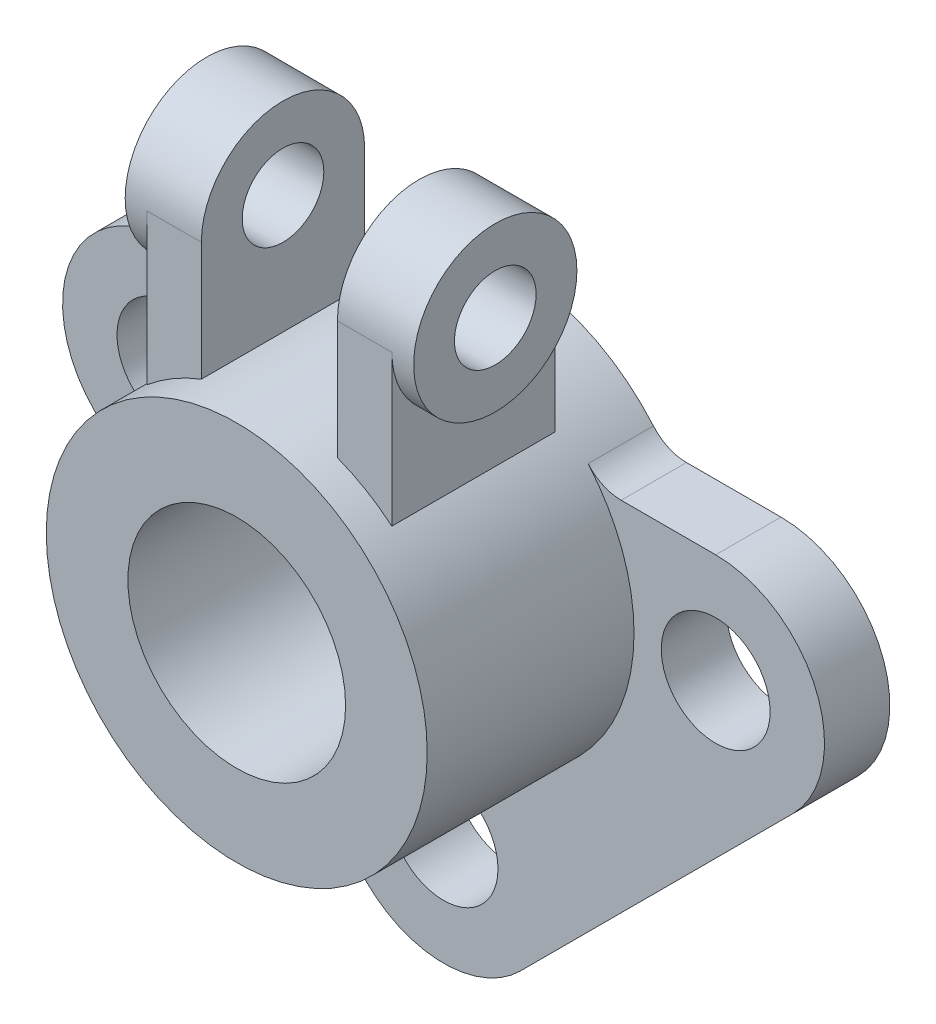
ISO-10303-21;
HEADER;
FILE_DESCRIPTION(('STEP AP214'),'2;1');
FILE_NAME('part.step','',(''),(''),'','','');
FILE_SCHEMA(('AUTOMOTIVE_DESIGN { 1 0 10303 214 1 1 1 1 }'));
ENDSEC;
DATA;
#1=APPLICATION_CONTEXT('core data for automotive mechanical design processes');
#2=APPLICATION_PROTOCOL_DEFINITION('international standard','automotive_design',2000,#1);
#3=PRODUCT_CONTEXT('',#1,'mechanical');
#4=PRODUCT('Part','Part','',(#3));
#5=PRODUCT_RELATED_PRODUCT_CATEGORY('part','',(#4));
#6=PRODUCT_DEFINITION_FORMATION('','',#4);
#7=PRODUCT_DEFINITION_CONTEXT('part definition',#1,'design');
#8=PRODUCT_DEFINITION('design','',#6,#7);
#9=PRODUCT_DEFINITION_SHAPE('','',#8);
#10=(LENGTH_UNIT() NAMED_UNIT(*) SI_UNIT(.MILLI.,.METRE.));
#11=(NAMED_UNIT(*) PLANE_ANGLE_UNIT() SI_UNIT($,.RADIAN.));
#12=(NAMED_UNIT(*) SI_UNIT($,.STERADIAN.) SOLID_ANGLE_UNIT());
#13=UNCERTAINTY_MEASURE_WITH_UNIT(LENGTH_MEASURE(1.E-05),#10,'distance_accuracy_value','');
#14=(GEOMETRIC_REPRESENTATION_CONTEXT(3) GLOBAL_UNCERTAINTY_ASSIGNED_CONTEXT((#13)) GLOBAL_UNIT_ASSIGNED_CONTEXT((#10,
#11,#12)) REPRESENTATION_CONTEXT('',''));
#15=CARTESIAN_POINT('',(0.,0.,0.));
#16=DIRECTION('',(0.,0.,1.));
#17=DIRECTION('',(1.,0.,0.));
#18=AXIS2_PLACEMENT_3D('',#15,#16,#17);
#19=CARTESIAN_POINT('',(-22.5,54.4714103742384,-21.));
#20=DIRECTION('',(1.,0.,0.));
#21=DIRECTION('',(0.,0.,-1.));
#22=AXIS2_PLACEMENT_3D('',#19,#20,#21);
#23=PLANE('',#22);
#24=CARTESIAN_POINT('',(-22.5,54.4714103742384,-21.));
#25=DIRECTION('',(1.,0.,0.));
#26=DIRECTION('',(0.,0.,-1.));
#27=AXIS2_PLACEMENT_3D('',#24,#25,#26);
#28=CIRCLE('',#27,15.);
#29=CARTESIAN_POINT('',(-22.5,54.4714103742384,-36.));
#30=VERTEX_POINT('',#29);
#31=CARTESIAN_POINT('',(-22.5,54.4714103742384,-6.00000000000001));
#32=VERTEX_POINT('',#31);
#33=EDGE_CURVE('E11',#30,#32,#28,.F.);
#34=ORIENTED_EDGE('',*,*,#33,.F.);
#35=DIRECTION('',(0.,1.,0.));
#36=VECTOR('',#35,1.);
#37=CARTESIAN_POINT('',(-22.5,54.4714103742384,-36.));
#38=LINE('',#37,#36);
#39=CARTESIAN_POINT('',(-22.5,26.809513236909,-36.));
#40=VERTEX_POINT('',#39);
#41=EDGE_CURVE('E168',#40,#30,#38,.T.);
#42=ORIENTED_EDGE('',*,*,#41,.F.);
#43=DIRECTION('',(0.,0.,1.));
#44=VECTOR('',#43,1.);
#45=CARTESIAN_POINT('',(-22.5,26.809513236909,-50.));
#46=LINE('',#45,#44);
#47=CARTESIAN_POINT('',(-22.5,26.809513236909,-6.00000000000001));
#48=VERTEX_POINT('',#47);
#49=EDGE_CURVE('E55',#48,#40,#46,.F.);
#50=ORIENTED_EDGE('',*,*,#49,.F.);
#51=DIRECTION('',(0.,-1.,0.));
#52=VECTOR('',#51,1.);
#53=CARTESIAN_POINT('',(-22.5,26.4714103742384,-6.00000000000001));
#54=LINE('',#53,#52);
#55=EDGE_CURVE('E166',#32,#48,#54,.T.);
#56=ORIENTED_EDGE('',*,*,#55,.F.);
#57=EDGE_LOOP('',(#34,#42,#50,#56));
#58=FACE_BOUND('',#57,.T.);
#59=ADVANCED_FACE('F43',(#58),#23,.F.);
#60=CARTESIAN_POINT('',(0.,0.,-50.));
#61=DIRECTION('',(0.,0.,1.));
#62=DIRECTION('',(1.,0.,0.));
#63=AXIS2_PLACEMENT_3D('',#60,#61,#62);
#64=CYLINDRICAL_SURFACE('',#63,35.);
#65=DIRECTION('',(0.,0.,1.));
#66=VECTOR('',#65,1.);
#67=CARTESIAN_POINT('',(22.5,26.809513236909,-50.));
#68=LINE('',#67,#66);
#69=CARTESIAN_POINT('',(22.5,26.809513236909,-6.));
#70=VERTEX_POINT('',#69);
#71=CARTESIAN_POINT('',(22.5,26.809513236909,-36.));
#72=VERTEX_POINT('',#71);
#73=EDGE_CURVE('E328',#70,#72,#68,.F.);
#74=ORIENTED_EDGE('',*,*,#73,.F.);
#75=CARTESIAN_POINT('',(0.,0.,-5.99999999999999));
#76=DIRECTION('',(0.,0.,-1.));
#77=DIRECTION('',(0.,1.,0.));
#78=AXIS2_PLACEMENT_3D('',#75,#76,#77);
#79=CIRCLE('',#78,35.);
#80=CARTESIAN_POINT('',(12.5,32.6917420765551,-6.));
#81=VERTEX_POINT('',#80);
#82=EDGE_CURVE('E324',#70,#81,#79,.F.);
#83=ORIENTED_EDGE('',*,*,#82,.T.);
#84=DIRECTION('',(0.,0.,1.));
#85=VECTOR('',#84,1.);
#86=CARTESIAN_POINT('',(12.5,32.6917420765551,-50.));
#87=LINE('',#86,#85);
#88=CARTESIAN_POINT('',(12.5,32.6917420765551,-36.));
#89=VERTEX_POINT('',#88);
#90=EDGE_CURVE('E320',#81,#89,#87,.F.);
#91=ORIENTED_EDGE('',*,*,#90,.T.);
#92=CARTESIAN_POINT('',(0.,0.,-36.));
#93=DIRECTION('',(0.,0.,1.));
#94=DIRECTION('',(0.,-1.,0.));
#95=AXIS2_PLACEMENT_3D('',#92,#93,#94);
#96=CIRCLE('',#95,35.);
#97=EDGE_CURVE('E318',#89,#72,#96,.F.);
#98=ORIENTED_EDGE('',*,*,#97,.T.);
#99=EDGE_LOOP('',(#74,#83,#91,#98));
#100=FACE_BOUND('',#99,.T.);
#101=CARTESIAN_POINT('',(0.,0.,-50.));
#102=DIRECTION('',(0.,0.,1.));
#103=DIRECTION('',(1.,0.,0.));
#104=AXIS2_PLACEMENT_3D('',#101,#102,#103);
#105=CIRCLE('',#104,35.);
#106=CARTESIAN_POINT('',(26.5628330475733,22.7906976744186,-50.));
#107=VERTEX_POINT('',#106);
#108=CARTESIAN_POINT('',(-26.5628330475733,22.7906976744186,-50.));
#109=VERTEX_POINT('',#108);
#110=EDGE_CURVE('E291',#107,#109,#105,.T.);
#111=ORIENTED_EDGE('',*,*,#110,.T.);
#112=DIRECTION('',(0.,0.,1.));
#113=VECTOR('',#112,1.);
#114=CARTESIAN_POINT('',(-26.5628330475733,22.7906976744186,-50.));
#115=LINE('',#114,#113);
#116=CARTESIAN_POINT('',(-26.5628330475733,22.7906976744186,-38.));
#117=VERTEX_POINT('',#116);
#118=EDGE_CURVE('E297',#109,#117,#115,.T.);
#119=ORIENTED_EDGE('',*,*,#118,.T.);
#120=CARTESIAN_POINT('',(0.,0.,-38.));
#121=DIRECTION('',(0.,0.,-1.));
#122=DIRECTION('',(1.,0.,0.));
#123=AXIS2_PLACEMENT_3D('',#120,#121,#122);
#124=CIRCLE('',#123,35.);
#125=CARTESIAN_POINT('',(26.5628330475733,22.7906976744186,-38.));
#126=VERTEX_POINT('',#125);
#127=EDGE_CURVE('E272',#126,#117,#124,.T.);
#128=ORIENTED_EDGE('',*,*,#127,.F.);
#129=DIRECTION('',(0.,0.,1.));
#130=VECTOR('',#129,1.);
#131=CARTESIAN_POINT('',(26.5628330475733,22.7906976744186,-50.));
#132=LINE('',#131,#130);
#133=EDGE_CURVE('E298',#126,#107,#132,.F.);
#134=ORIENTED_EDGE('',*,*,#133,.T.);
#135=EDGE_LOOP('',(#111,#119,#128,#134));
#136=FACE_BOUND('',#135,.T.);
#137=CARTESIAN_POINT('',(0.,0.,0.));
#138=DIRECTION('',(0.,0.,1.));
#139=DIRECTION('',(1.,0.,0.));
#140=AXIS2_PLACEMENT_3D('',#137,#138,#139);
#141=CIRCLE('',#140,35.);
#142=CARTESIAN_POINT('',(35.,0.,0.));
#143=VERTEX_POINT('',#142);
#144=EDGE_CURVE('E287',#143,#143,#141,.T.);
#145=ORIENTED_EDGE('',*,*,#144,.F.);
#146=EDGE_LOOP('',(#145));
#147=FACE_BOUND('',#146,.T.);
#148=CARTESIAN_POINT('',(0.,0.,-6.00000000000001));
#149=DIRECTION('',(0.,0.,1.));
#150=DIRECTION('',(0.,-1.,0.));
#151=AXIS2_PLACEMENT_3D('',#148,#149,#150);
#152=CIRCLE('',#151,35.);
#153=CARTESIAN_POINT('',(-12.5,32.6917420765551,-6.00000000000001));
#154=VERTEX_POINT('',#153);
#155=EDGE_CURVE('E64',#48,#154,#152,.F.);
#156=ORIENTED_EDGE('',*,*,#155,.F.);
#157=ORIENTED_EDGE('',*,*,#49,.T.);
#158=CARTESIAN_POINT('',(0.,0.,-36.));
#159=DIRECTION('',(0.,0.,-1.));
#160=DIRECTION('',(0.,1.,0.));
#161=AXIS2_PLACEMENT_3D('',#158,#159,#160);
#162=CIRCLE('',#161,35.);
#163=CARTESIAN_POINT('',(-12.5,32.6917420765551,-36.));
#164=VERTEX_POINT('',#163);
#165=EDGE_CURVE('E178',#164,#40,#162,.F.);
#166=ORIENTED_EDGE('',*,*,#165,.F.);
#167=DIRECTION('',(0.,0.,1.));
#168=VECTOR('',#167,1.);
#169=CARTESIAN_POINT('',(-12.5,32.6917420765551,-50.));
#170=LINE('',#169,#168);
#171=EDGE_CURVE('E333',#154,#164,#170,.F.);
#172=ORIENTED_EDGE('',*,*,#171,.F.);
#173=EDGE_LOOP('',(#156,#157,#166,#172));
#174=FACE_BOUND('',#173,.T.);
#175=ADVANCED_FACE('F385',(#100,#136,#147,#174),#64,.T.);
#176=CARTESIAN_POINT('',(22.5,54.4714103742384,-21.));
#177=DIRECTION('',(1.,0.,0.));
#178=DIRECTION('',(0.,0.,-1.));
#179=AXIS2_PLACEMENT_3D('',#176,#177,#178);
#180=PLANE('',#179);
#181=DIRECTION('',(0.,1.,0.));
#182=VECTOR('',#181,1.);
#183=CARTESIAN_POINT('',(22.5,26.4714103742384,-36.));
#184=LINE('',#183,#182);
#185=CARTESIAN_POINT('',(22.5,54.4714103742384,-36.));
#186=VERTEX_POINT('',#185);
#187=EDGE_CURVE('E197',#72,#186,#184,.T.);
#188=ORIENTED_EDGE('',*,*,#187,.T.);
#189=CARTESIAN_POINT('',(22.5,54.4714103742384,-21.));
#190=DIRECTION('',(1.,0.,0.));
#191=DIRECTION('',(0.,0.,-1.));
#192=AXIS2_PLACEMENT_3D('',#189,#190,#191);
#193=CIRCLE('',#192,15.);
#194=CARTESIAN_POINT('',(22.5,54.4714103742384,-6.00000000000001));
#195=VERTEX_POINT('',#194);
#196=EDGE_CURVE('E327',#186,#195,#193,.F.);
#197=ORIENTED_EDGE('',*,*,#196,.T.);
#198=DIRECTION('',(0.,-1.,0.));
#199=VECTOR('',#198,1.);
#200=CARTESIAN_POINT('',(22.5,54.4714103742384,-6.00000000000001));
#201=LINE('',#200,#199);
#202=EDGE_CURVE('E193',#195,#70,#201,.T.);
#203=ORIENTED_EDGE('',*,*,#202,.T.);
#204=ORIENTED_EDGE('',*,*,#73,.T.);
#205=EDGE_LOOP('',(#188,#197,#203,#204));
#206=FACE_BOUND('',#205,.T.);
#207=ADVANCED_FACE('F390',(#206),#180,.T.);
#208=CARTESIAN_POINT('',(0.,0.,-50.));
#209=DIRECTION('',(0.,0.,1.));
#210=DIRECTION('',(1.,0.,0.));
#211=AXIS2_PLACEMENT_3D('',#208,#209,#210);
#212=PLANE('',#211);
#213=CARTESIAN_POINT('',(50.,0.,-50.));
#214=DIRECTION('',(0.,0.,1.));
#215=DIRECTION('',(1.,0.,0.));
#216=AXIS2_PLACEMENT_3D('',#213,#214,#215);
#217=CIRCLE('',#216,10.);
#218=CARTESIAN_POINT('',(60.,0.,-50.));
#219=VERTEX_POINT('',#218);
#220=EDGE_CURVE('E211',#219,#219,#217,.T.);
#221=ORIENTED_EDGE('',*,*,#220,.T.);
#222=EDGE_LOOP('',(#221));
#223=FACE_BOUND('',#222,.T.);
#224=CARTESIAN_POINT('',(0.,-50.,-50.));
#225=DIRECTION('',(0.,0.,1.));
#226=DIRECTION('',(1.,0.,0.));
#227=AXIS2_PLACEMENT_3D('',#224,#225,#226);
#228=CIRCLE('',#227,10.);
#229=CARTESIAN_POINT('',(10.,-50.,-50.));
#230=VERTEX_POINT('',#229);
#231=EDGE_CURVE('E223',#230,#230,#228,.T.);
#232=ORIENTED_EDGE('',*,*,#231,.T.);
#233=EDGE_LOOP('',(#232));
#234=FACE_BOUND('',#233,.T.);
#235=CARTESIAN_POINT('',(-50.,0.,-50.));
#236=DIRECTION('',(0.,0.,1.));
#237=DIRECTION('',(1.,0.,0.));
#238=AXIS2_PLACEMENT_3D('',#235,#236,#237);
#239=CIRCLE('',#238,10.);
#240=CARTESIAN_POINT('',(-40.,0.,-50.));
#241=VERTEX_POINT('',#240);
#242=EDGE_CURVE('E227',#241,#241,#239,.T.);
#243=ORIENTED_EDGE('',*,*,#242,.T.);
#244=EDGE_LOOP('',(#243));
#245=FACE_BOUND('',#244,.T.);
#246=CARTESIAN_POINT('',(0.,0.,-50.));
#247=DIRECTION('',(0.,0.,1.));
#248=DIRECTION('',(1.,0.,0.));
#249=AXIS2_PLACEMENT_3D('',#246,#247,#248);
#250=CIRCLE('',#249,20.);
#251=CARTESIAN_POINT('',(20.,0.,-50.));
#252=VERTEX_POINT('',#251);
#253=EDGE_CURVE('E290',#252,#252,#250,.T.);
#254=ORIENTED_EDGE('',*,*,#253,.T.);
#255=EDGE_LOOP('',(#254));
#256=FACE_BOUND('',#255,.T.);
#257=ORIENTED_EDGE('',*,*,#110,.F.);
#258=CARTESIAN_POINT('',(32.6343377441614,28.,-50.));
#259=DIRECTION('',(0.,0.,1.));
#260=DIRECTION('',(1.,0.,0.));
#261=AXIS2_PLACEMENT_3D('',#258,#259,#260);
#262=CIRCLE('',#261,8.);
#263=CARTESIAN_POINT('',(32.6343377441614,20.,-50.));
#264=VERTEX_POINT('',#263);
#265=EDGE_CURVE('E314',#107,#264,#262,.T.);
#266=ORIENTED_EDGE('',*,*,#265,.T.);
#267=DIRECTION('',(-1.,0.,0.));
#268=VECTOR('',#267,1.);
#269=CARTESIAN_POINT('',(50.,20.,-50.));
#270=LINE('',#269,#268);
#271=CARTESIAN_POINT('',(50.,20.,-50.));
#272=VERTEX_POINT('',#271);
#273=EDGE_CURVE('E247',#272,#264,#270,.T.);
#274=ORIENTED_EDGE('',*,*,#273,.F.);
#275=CARTESIAN_POINT('',(50.,0.,-50.));
#276=DIRECTION('',(0.,0.,1.));
#277=DIRECTION('',(1.,0.,0.));
#278=AXIS2_PLACEMENT_3D('',#275,#276,#277);
#279=CIRCLE('',#278,20.);
#280=CARTESIAN_POINT('',(64.1421356237309,-14.142135623731,-50.));
#281=VERTEX_POINT('',#280);
#282=EDGE_CURVE('E244',#281,#272,#279,.T.);
#283=ORIENTED_EDGE('',*,*,#282,.F.);
#284=DIRECTION('',(0.707106781186547,0.707106781186548,0.));
#285=VECTOR('',#284,1.);
#286=CARTESIAN_POINT('',(64.142135623731,-14.1421356237309,-50.));
#287=LINE('',#286,#285);
#288=CARTESIAN_POINT('',(14.142135623731,-64.142135623731,-50.));
#289=VERTEX_POINT('',#288);
#290=EDGE_CURVE('E245',#289,#281,#287,.T.);
#291=ORIENTED_EDGE('',*,*,#290,.F.);
#292=CARTESIAN_POINT('',(0.,-50.,-50.));
#293=DIRECTION('',(0.,0.,1.));
#294=DIRECTION('',(1.,0.,0.));
#295=AXIS2_PLACEMENT_3D('',#292,#293,#294);
#296=CIRCLE('',#295,20.);
#297=CARTESIAN_POINT('',(-14.142135623731,-64.142135623731,-50.));
#298=VERTEX_POINT('',#297);
#299=EDGE_CURVE('E237',#298,#289,#296,.T.);
#300=ORIENTED_EDGE('',*,*,#299,.F.);
#301=DIRECTION('',(0.707106781186547,-0.707106781186547,0.));
#302=VECTOR('',#301,1.);
#303=CARTESIAN_POINT('',(-64.142135623731,-14.142135623731,-50.));
#304=LINE('',#303,#302);
#305=CARTESIAN_POINT('',(-64.142135623731,-14.142135623731,-50.));
#306=VERTEX_POINT('',#305);
#307=EDGE_CURVE('E232',#306,#298,#304,.T.);
#308=ORIENTED_EDGE('',*,*,#307,.F.);
#309=CARTESIAN_POINT('',(-50.,0.,-50.));
#310=DIRECTION('',(0.,0.,1.));
#311=DIRECTION('',(1.,0.,0.));
#312=AXIS2_PLACEMENT_3D('',#309,#310,#311);
#313=CIRCLE('',#312,20.);
#314=CARTESIAN_POINT('',(-50.,20.,-50.));
#315=VERTEX_POINT('',#314);
#316=EDGE_CURVE('E235',#315,#306,#313,.T.);
#317=ORIENTED_EDGE('',*,*,#316,.F.);
#318=DIRECTION('',(-1.,0.,0.));
#319=VECTOR('',#318,1.);
#320=CARTESIAN_POINT('',(-50.,20.,-50.));
#321=LINE('',#320,#319);
#322=CARTESIAN_POINT('',(-32.6343377441614,20.,-50.));
#323=VERTEX_POINT('',#322);
#324=EDGE_CURVE('E252',#323,#315,#321,.T.);
#325=ORIENTED_EDGE('',*,*,#324,.F.);
#326=CARTESIAN_POINT('',(-32.6343377441614,28.,-50.));
#327=DIRECTION('',(0.,0.,1.));
#328=DIRECTION('',(1.,0.,0.));
#329=AXIS2_PLACEMENT_3D('',#326,#327,#328);
#330=CIRCLE('',#329,8.);
#331=EDGE_CURVE('E309',#323,#109,#330,.T.);
#332=ORIENTED_EDGE('',*,*,#331,.T.);
#333=EDGE_LOOP('',(#257,#266,#274,#283,#291,#300,#308,#317,#325,#332));
#334=FACE_BOUND('',#333,.T.);
#335=ADVANCED_FACE('F579',(#223,#234,#245,#256,#334),#212,.F.);
#336=CARTESIAN_POINT('',(0.,0.,0.));
#337=DIRECTION('',(0.,0.,1.));
#338=DIRECTION('',(1.,0.,0.));
#339=AXIS2_PLACEMENT_3D('',#336,#337,#338);
#340=PLANE('',#339);
#341=CARTESIAN_POINT('',(0.,0.,0.));
#342=DIRECTION('',(0.,0.,1.));
#343=DIRECTION('',(1.,0.,0.));
#344=AXIS2_PLACEMENT_3D('',#341,#342,#343);
#345=CIRCLE('',#344,20.);
#346=CARTESIAN_POINT('',(20.,0.,0.));
#347=VERTEX_POINT('',#346);
#348=EDGE_CURVE('E280',#347,#347,#345,.T.);
#349=ORIENTED_EDGE('',*,*,#348,.F.);
#350=EDGE_LOOP('',(#349));
#351=FACE_BOUND('',#350,.T.);
#352=ORIENTED_EDGE('',*,*,#144,.T.);
#353=EDGE_LOOP('',(#352));
#354=FACE_BOUND('',#353,.T.);
#355=ADVANCED_FACE('F481',(#351,#354),#340,.T.);
#356=CARTESIAN_POINT('',(0.,0.,-50.));
#357=DIRECTION('',(0.,0.,1.));
#358=DIRECTION('',(1.,0.,0.));
#359=AXIS2_PLACEMENT_3D('',#356,#357,#358);
#360=CYLINDRICAL_SURFACE('',#359,20.);
#361=ORIENTED_EDGE('',*,*,#253,.F.);
#362=EDGE_LOOP('',(#361));
#363=FACE_BOUND('',#362,.T.);
#364=ORIENTED_EDGE('',*,*,#348,.T.);
#365=EDGE_LOOP('',(#364));
#366=FACE_BOUND('',#365,.T.);
#367=ADVANCED_FACE('F476',(#363,#366),#360,.F.);
#368=CARTESIAN_POINT('',(-50.,0.,-50.));
#369=DIRECTION('',(0.,0.,1.));
#370=DIRECTION('',(1.,0.,0.));
#371=AXIS2_PLACEMENT_3D('',#368,#369,#370);
#372=CYLINDRICAL_SURFACE('',#371,20.);
#373=CARTESIAN_POINT('',(-50.,0.,-38.));
#374=DIRECTION('',(0.,0.,1.));
#375=DIRECTION('',(1.,0.,0.));
#376=AXIS2_PLACEMENT_3D('',#373,#374,#375);
#377=CIRCLE('',#376,20.);
#378=CARTESIAN_POINT('',(-50.,20.,-38.));
#379=VERTEX_POINT('',#378);
#380=CARTESIAN_POINT('',(-64.142135623731,-14.142135623731,-38.));
#381=VERTEX_POINT('',#380);
#382=EDGE_CURVE('E219',#379,#381,#377,.T.);
#383=ORIENTED_EDGE('',*,*,#382,.F.);
#384=DIRECTION('',(0.,0.,1.));
#385=VECTOR('',#384,1.);
#386=CARTESIAN_POINT('',(-50.,20.,-50.));
#387=LINE('',#386,#385);
#388=EDGE_CURVE('E274',#315,#379,#387,.T.);
#389=ORIENTED_EDGE('',*,*,#388,.F.);
#390=ORIENTED_EDGE('',*,*,#316,.T.);
#391=DIRECTION('',(0.,0.,1.));
#392=VECTOR('',#391,1.);
#393=CARTESIAN_POINT('',(-64.142135623731,-14.142135623731,-50.));
#394=LINE('',#393,#392);
#395=EDGE_CURVE('E254',#306,#381,#394,.T.);
#396=ORIENTED_EDGE('',*,*,#395,.T.);
#397=EDGE_LOOP('',(#383,#389,#390,#396));
#398=FACE_BOUND('',#397,.T.);
#399=ADVANCED_FACE('F485',(#398),#372,.T.);
#400=CARTESIAN_POINT('',(-50.,20.,-50.));
#401=DIRECTION('',(0.,1.,0.));
#402=DIRECTION('',(0.,0.,1.));
#403=AXIS2_PLACEMENT_3D('',#400,#401,#402);
#404=PLANE('',#403);
#405=DIRECTION('',(-1.,0.,0.));
#406=VECTOR('',#405,1.);
#407=CARTESIAN_POINT('',(-50.,20.,-38.));
#408=LINE('',#407,#406);
#409=CARTESIAN_POINT('',(-32.6343377441614,20.,-38.));
#410=VERTEX_POINT('',#409);
#411=EDGE_CURVE('E236',#410,#379,#408,.T.);
#412=ORIENTED_EDGE('',*,*,#411,.F.);
#413=DIRECTION('',(0.,0.,-1.));
#414=VECTOR('',#413,1.);
#415=CARTESIAN_POINT('',(-32.6343377441614,20.,-50.));
#416=LINE('',#415,#414);
#417=EDGE_CURVE('E303',#410,#323,#416,.T.);
#418=ORIENTED_EDGE('',*,*,#417,.T.);
#419=ORIENTED_EDGE('',*,*,#324,.T.);
#420=ORIENTED_EDGE('',*,*,#388,.T.);
#421=EDGE_LOOP('',(#412,#418,#419,#420));
#422=FACE_BOUND('',#421,.T.);
#423=ADVANCED_FACE('F501',(#422),#404,.T.);
#424=CARTESIAN_POINT('',(50.,20.,-50.));
#425=DIRECTION('',(0.,1.,0.));
#426=DIRECTION('',(-1.,0.,0.));
#427=AXIS2_PLACEMENT_3D('',#424,#425,#426);
#428=PLANE('',#427);
#429=ORIENTED_EDGE('',*,*,#273,.T.);
#430=DIRECTION('',(0.,0.,-1.));
#431=VECTOR('',#430,1.);
#432=CARTESIAN_POINT('',(32.6343377441614,20.,-38.));
#433=LINE('',#432,#431);
#434=CARTESIAN_POINT('',(32.6343377441614,20.,-38.));
#435=VERTEX_POINT('',#434);
#436=EDGE_CURVE('E304',#264,#435,#433,.F.);
#437=ORIENTED_EDGE('',*,*,#436,.T.);
#438=DIRECTION('',(-1.,0.,0.));
#439=VECTOR('',#438,1.);
#440=CARTESIAN_POINT('',(50.,20.,-38.));
#441=LINE('',#440,#439);
#442=CARTESIAN_POINT('',(50.,20.,-38.));
#443=VERTEX_POINT('',#442);
#444=EDGE_CURVE('E266',#443,#435,#441,.T.);
#445=ORIENTED_EDGE('',*,*,#444,.F.);
#446=DIRECTION('',(0.,0.,1.));
#447=VECTOR('',#446,1.);
#448=CARTESIAN_POINT('',(50.,20.,-50.));
#449=LINE('',#448,#447);
#450=EDGE_CURVE('E279',#272,#443,#449,.T.);
#451=ORIENTED_EDGE('',*,*,#450,.F.);
#452=EDGE_LOOP('',(#429,#437,#445,#451));
#453=FACE_BOUND('',#452,.T.);
#454=ADVANCED_FACE('F514',(#453),#428,.T.);
#455=CARTESIAN_POINT('',(50.,0.,-50.));
#456=DIRECTION('',(0.,0.,1.));
#457=DIRECTION('',(1.,0.,0.));
#458=AXIS2_PLACEMENT_3D('',#455,#456,#457);
#459=CYLINDRICAL_SURFACE('',#458,20.);
#460=CARTESIAN_POINT('',(50.,0.,-38.));
#461=DIRECTION('',(0.,0.,1.));
#462=DIRECTION('',(1.,0.,0.));
#463=AXIS2_PLACEMENT_3D('',#460,#461,#462);
#464=CIRCLE('',#463,20.);
#465=CARTESIAN_POINT('',(64.1421356237309,-14.142135623731,-38.));
#466=VERTEX_POINT('',#465);
#467=EDGE_CURVE('E261',#466,#443,#464,.T.);
#468=ORIENTED_EDGE('',*,*,#467,.F.);
#469=DIRECTION('',(0.,0.,1.));
#470=VECTOR('',#469,1.);
#471=CARTESIAN_POINT('',(64.1421356237309,-14.142135623731,-50.));
#472=LINE('',#471,#470);
#473=EDGE_CURVE('E278',#281,#466,#472,.T.);
#474=ORIENTED_EDGE('',*,*,#473,.F.);
#475=ORIENTED_EDGE('',*,*,#282,.T.);
#476=ORIENTED_EDGE('',*,*,#450,.T.);
#477=EDGE_LOOP('',(#468,#474,#475,#476));
#478=FACE_BOUND('',#477,.T.);
#479=ADVANCED_FACE('F507',(#478),#459,.T.);
#480=CARTESIAN_POINT('',(64.142135623731,-14.1421356237309,-50.));
#481=DIRECTION('',(0.707106781186548,-0.707106781186547,0.));
#482=DIRECTION('',(0.707106781186547,0.707106781186548,0.));
#483=AXIS2_PLACEMENT_3D('',#480,#481,#482);
#484=PLANE('',#483);
#485=DIRECTION('',(0.707106781186547,0.707106781186548,0.));
#486=VECTOR('',#485,1.);
#487=CARTESIAN_POINT('',(64.142135623731,-14.1421356237309,-38.));
#488=LINE('',#487,#486);
#489=CARTESIAN_POINT('',(14.142135623731,-64.142135623731,-38.));
#490=VERTEX_POINT('',#489);
#491=EDGE_CURVE('E264',#490,#466,#488,.T.);
#492=ORIENTED_EDGE('',*,*,#491,.F.);
#493=DIRECTION('',(0.,0.,1.));
#494=VECTOR('',#493,1.);
#495=CARTESIAN_POINT('',(14.142135623731,-64.142135623731,-50.));
#496=LINE('',#495,#494);
#497=EDGE_CURVE('E284',#289,#490,#496,.T.);
#498=ORIENTED_EDGE('',*,*,#497,.F.);
#499=ORIENTED_EDGE('',*,*,#290,.T.);
#500=ORIENTED_EDGE('',*,*,#473,.T.);
#501=EDGE_LOOP('',(#492,#498,#499,#500));
#502=FACE_BOUND('',#501,.T.);
#503=ADVANCED_FACE('F515',(#502),#484,.T.);
#504=CARTESIAN_POINT('',(0.,-50.,-50.));
#505=DIRECTION('',(0.,0.,1.));
#506=DIRECTION('',(1.,0.,0.));
#507=AXIS2_PLACEMENT_3D('',#504,#505,#506);
#508=CYLINDRICAL_SURFACE('',#507,20.);
#509=CARTESIAN_POINT('',(0.,-50.,-38.));
#510=DIRECTION('',(0.,0.,1.));
#511=DIRECTION('',(1.,0.,0.));
#512=AXIS2_PLACEMENT_3D('',#509,#510,#511);
#513=CIRCLE('',#512,20.);
#514=CARTESIAN_POINT('',(-14.142135623731,-64.142135623731,-38.));
#515=VERTEX_POINT('',#514);
#516=EDGE_CURVE('E256',#515,#490,#513,.T.);
#517=ORIENTED_EDGE('',*,*,#516,.F.);
#518=DIRECTION('',(0.,0.,1.));
#519=VECTOR('',#518,1.);
#520=CARTESIAN_POINT('',(-14.142135623731,-64.142135623731,-50.));
#521=LINE('',#520,#519);
#522=EDGE_CURVE('E285',#298,#515,#521,.T.);
#523=ORIENTED_EDGE('',*,*,#522,.F.);
#524=ORIENTED_EDGE('',*,*,#299,.T.);
#525=ORIENTED_EDGE('',*,*,#497,.T.);
#526=EDGE_LOOP('',(#517,#523,#524,#525));
#527=FACE_BOUND('',#526,.T.);
#528=ADVANCED_FACE('F522',(#527),#508,.T.);
#529=CARTESIAN_POINT('',(-64.142135623731,-14.142135623731,-50.));
#530=DIRECTION('',(-0.707106781186547,-0.707106781186548,0.));
#531=DIRECTION('',(0.707106781186548,-0.707106781186547,0.));
#532=AXIS2_PLACEMENT_3D('',#529,#530,#531);
#533=PLANE('',#532);
#534=DIRECTION('',(0.707106781186547,-0.707106781186547,0.));
#535=VECTOR('',#534,1.);
#536=CARTESIAN_POINT('',(-64.142135623731,-14.142135623731,-38.));
#537=LINE('',#536,#535);
#538=EDGE_CURVE('E257',#381,#515,#537,.T.);
#539=ORIENTED_EDGE('',*,*,#538,.F.);
#540=ORIENTED_EDGE('',*,*,#395,.F.);
#541=ORIENTED_EDGE('',*,*,#307,.T.);
#542=ORIENTED_EDGE('',*,*,#522,.T.);
#543=EDGE_LOOP('',(#539,#540,#541,#542));
#544=FACE_BOUND('',#543,.T.);
#545=ADVANCED_FACE('F535',(#544),#533,.T.);
#546=CARTESIAN_POINT('',(-50.,0.,-38.));
#547=DIRECTION('',(0.,0.,1.));
#548=DIRECTION('',(1.,0.,0.));
#549=AXIS2_PLACEMENT_3D('',#546,#547,#548);
#550=PLANE('',#549);
#551=CARTESIAN_POINT('',(50.,0.,-38.));
#552=DIRECTION('',(0.,0.,1.));
#553=DIRECTION('',(1.,0.,0.));
#554=AXIS2_PLACEMENT_3D('',#551,#552,#553);
#555=CIRCLE('',#554,10.);
#556=CARTESIAN_POINT('',(60.,0.,-38.));
#557=VERTEX_POINT('',#556);
#558=EDGE_CURVE('E217',#557,#557,#555,.T.);
#559=ORIENTED_EDGE('',*,*,#558,.F.);
#560=EDGE_LOOP('',(#559));
#561=FACE_BOUND('',#560,.T.);
#562=CARTESIAN_POINT('',(0.,-50.,-38.));
#563=DIRECTION('',(0.,0.,1.));
#564=DIRECTION('',(1.,0.,0.));
#565=AXIS2_PLACEMENT_3D('',#562,#563,#564);
#566=CIRCLE('',#565,10.);
#567=CARTESIAN_POINT('',(10.,-50.,-38.));
#568=VERTEX_POINT('',#567);
#569=EDGE_CURVE('E224',#568,#568,#566,.T.);
#570=ORIENTED_EDGE('',*,*,#569,.F.);
#571=EDGE_LOOP('',(#570));
#572=FACE_BOUND('',#571,.T.);
#573=CARTESIAN_POINT('',(-50.,0.,-38.));
#574=DIRECTION('',(0.,0.,1.));
#575=DIRECTION('',(1.,0.,0.));
#576=AXIS2_PLACEMENT_3D('',#573,#574,#575);
#577=CIRCLE('',#576,10.);
#578=CARTESIAN_POINT('',(-40.,0.,-38.));
#579=VERTEX_POINT('',#578);
#580=EDGE_CURVE('E214',#579,#579,#577,.T.);
#581=ORIENTED_EDGE('',*,*,#580,.F.);
#582=EDGE_LOOP('',(#581));
#583=FACE_BOUND('',#582,.T.);
#584=ORIENTED_EDGE('',*,*,#382,.T.);
#585=ORIENTED_EDGE('',*,*,#538,.T.);
#586=ORIENTED_EDGE('',*,*,#516,.T.);
#587=ORIENTED_EDGE('',*,*,#491,.T.);
#588=ORIENTED_EDGE('',*,*,#467,.T.);
#589=ORIENTED_EDGE('',*,*,#444,.T.);
#590=CARTESIAN_POINT('',(32.6343377441614,28.,-38.));
#591=DIRECTION('',(0.,0.,1.));
#592=DIRECTION('',(1.,0.,0.));
#593=AXIS2_PLACEMENT_3D('',#590,#591,#592);
#594=CIRCLE('',#593,8.);
#595=EDGE_CURVE('E315',#435,#126,#594,.F.);
#596=ORIENTED_EDGE('',*,*,#595,.T.);
#597=ORIENTED_EDGE('',*,*,#127,.T.);
#598=CARTESIAN_POINT('',(-32.6343377441614,28.,-38.));
#599=DIRECTION('',(0.,0.,1.));
#600=DIRECTION('',(1.,0.,0.));
#601=AXIS2_PLACEMENT_3D('',#598,#599,#600);
#602=CIRCLE('',#601,8.);
#603=EDGE_CURVE('E308',#117,#410,#602,.F.);
#604=ORIENTED_EDGE('',*,*,#603,.T.);
#605=ORIENTED_EDGE('',*,*,#411,.T.);
#606=EDGE_LOOP('',(#584,#585,#586,#587,#588,#589,#596,#597,#604,#605));
#607=FACE_BOUND('',#606,.T.);
#608=ADVANCED_FACE('F543',(#561,#572,#583,#607),#550,.T.);
#609=CARTESIAN_POINT('',(-32.6343377441614,28.,-50.));
#610=DIRECTION('',(0.,0.,1.));
#611=DIRECTION('',(1.,0.,0.));
#612=AXIS2_PLACEMENT_3D('',#609,#610,#611);
#613=CYLINDRICAL_SURFACE('',#612,8.);
#614=ORIENTED_EDGE('',*,*,#331,.F.);
#615=ORIENTED_EDGE('',*,*,#417,.F.);
#616=ORIENTED_EDGE('',*,*,#603,.F.);
#617=ORIENTED_EDGE('',*,*,#118,.F.);
#618=EDGE_LOOP('',(#614,#615,#616,#617));
#619=FACE_BOUND('',#618,.T.);
#620=ADVANCED_FACE('F565',(#619),#613,.F.);
#621=CARTESIAN_POINT('',(32.6343377441614,28.,-50.));
#622=DIRECTION('',(0.,0.,1.));
#623=DIRECTION('',(1.,0.,0.));
#624=AXIS2_PLACEMENT_3D('',#621,#622,#623);
#625=CYLINDRICAL_SURFACE('',#624,8.);
#626=ORIENTED_EDGE('',*,*,#265,.F.);
#627=ORIENTED_EDGE('',*,*,#133,.F.);
#628=ORIENTED_EDGE('',*,*,#595,.F.);
#629=ORIENTED_EDGE('',*,*,#436,.F.);
#630=EDGE_LOOP('',(#626,#627,#628,#629));
#631=FACE_BOUND('',#630,.T.);
#632=ADVANCED_FACE('F44',(#631),#625,.F.);
#633=CARTESIAN_POINT('',(-50.,0.,-50.));
#634=DIRECTION('',(0.,0.,1.));
#635=DIRECTION('',(1.,0.,0.));
#636=AXIS2_PLACEMENT_3D('',#633,#634,#635);
#637=CYLINDRICAL_SURFACE('',#636,10.);
#638=ORIENTED_EDGE('',*,*,#242,.F.);
#639=EDGE_LOOP('',(#638));
#640=FACE_BOUND('',#639,.T.);
#641=ORIENTED_EDGE('',*,*,#580,.T.);
#642=EDGE_LOOP('',(#641));
#643=FACE_BOUND('',#642,.T.);
#644=ADVANCED_FACE('F470',(#640,#643),#637,.F.);
#645=CARTESIAN_POINT('',(0.,-50.,-50.));
#646=DIRECTION('',(0.,0.,1.));
#647=DIRECTION('',(1.,0.,0.));
#648=AXIS2_PLACEMENT_3D('',#645,#646,#647);
#649=CYLINDRICAL_SURFACE('',#648,10.);
#650=ORIENTED_EDGE('',*,*,#231,.F.);
#651=EDGE_LOOP('',(#650));
#652=FACE_BOUND('',#651,.T.);
#653=ORIENTED_EDGE('',*,*,#569,.T.);
#654=EDGE_LOOP('',(#653));
#655=FACE_BOUND('',#654,.T.);
#656=ADVANCED_FACE('F460',(#652,#655),#649,.F.);
#657=CARTESIAN_POINT('',(50.,0.,-50.));
#658=DIRECTION('',(0.,0.,1.));
#659=DIRECTION('',(1.,0.,0.));
#660=AXIS2_PLACEMENT_3D('',#657,#658,#659);
#661=CYLINDRICAL_SURFACE('',#660,10.);
#662=ORIENTED_EDGE('',*,*,#220,.F.);
#663=EDGE_LOOP('',(#662));
#664=FACE_BOUND('',#663,.T.);
#665=ORIENTED_EDGE('',*,*,#558,.T.);
#666=EDGE_LOOP('',(#665));
#667=FACE_BOUND('',#666,.T.);
#668=ADVANCED_FACE('F453',(#664,#667),#661,.F.);
#669=CARTESIAN_POINT('',(22.5,54.4714103742384,-21.));
#670=DIRECTION('',(-1.,0.,0.));
#671=DIRECTION('',(0.,0.,1.));
#672=AXIS2_PLACEMENT_3D('',#669,#670,#671);
#673=CYLINDRICAL_SURFACE('',#672,15.);
#674=CARTESIAN_POINT('',(12.5,54.4714103742384,-21.));
#675=DIRECTION('',(1.,0.,0.));
#676=DIRECTION('',(0.,0.,-1.));
#677=AXIS2_PLACEMENT_3D('',#674,#675,#676);
#678=CIRCLE('',#677,15.);
#679=CARTESIAN_POINT('',(12.5,54.4714103742384,-36.));
#680=VERTEX_POINT('',#679);
#681=CARTESIAN_POINT('',(12.5,54.4714103742384,-6.00000000000001));
#682=VERTEX_POINT('',#681);
#683=EDGE_CURVE('E189',#680,#682,#678,.T.);
#684=ORIENTED_EDGE('',*,*,#683,.T.);
#685=DIRECTION('',(-1.,0.,0.));
#686=VECTOR('',#685,1.);
#687=CARTESIAN_POINT('',(22.5,54.4714103742384,-6.00000000000001));
#688=LINE('',#687,#686);
#689=EDGE_CURVE('E208',#195,#682,#688,.T.);
#690=ORIENTED_EDGE('',*,*,#689,.F.);
#691=ORIENTED_EDGE('',*,*,#196,.F.);
#692=DIRECTION('',(-1.,0.,0.));
#693=VECTOR('',#692,1.);
#694=CARTESIAN_POINT('',(22.5,54.4714103742384,-36.));
#695=LINE('',#694,#693);
#696=EDGE_CURVE('E203',#186,#680,#695,.T.);
#697=ORIENTED_EDGE('',*,*,#696,.T.);
#698=EDGE_LOOP('',(#684,#690,#691,#697));
#699=FACE_BOUND('',#698,.T.);
#700=CARTESIAN_POINT('',(26.5,54.4714103742384,-21.));
#701=DIRECTION('',(1.,0.,0.));
#702=DIRECTION('',(0.,0.,-1.));
#703=AXIS2_PLACEMENT_3D('',#700,#701,#702);
#704=CIRCLE('',#703,15.);
#705=CARTESIAN_POINT('',(26.5,54.4714103742384,-36.));
#706=VERTEX_POINT('',#705);
#707=EDGE_CURVE('E184',#706,#706,#704,.T.);
#708=ORIENTED_EDGE('',*,*,#707,.F.);
#709=EDGE_LOOP('',(#708));
#710=FACE_BOUND('',#709,.T.);
#711=ADVANCED_FACE('F457',(#699,#710),#673,.T.);
#712=CARTESIAN_POINT('',(22.5,54.4714103742384,-6.00000000000001));
#713=DIRECTION('',(0.,0.,-1.));
#714=DIRECTION('',(0.,1.,0.));
#715=AXIS2_PLACEMENT_3D('',#712,#713,#714);
#716=PLANE('',#715);
#717=ORIENTED_EDGE('',*,*,#82,.F.);
#718=ORIENTED_EDGE('',*,*,#202,.F.);
#719=ORIENTED_EDGE('',*,*,#689,.T.);
#720=DIRECTION('',(0.,-1.,0.));
#721=VECTOR('',#720,1.);
#722=CARTESIAN_POINT('',(12.5,54.4714103742384,-6.00000000000001));
#723=LINE('',#722,#721);
#724=EDGE_CURVE('E204',#682,#81,#723,.T.);
#725=ORIENTED_EDGE('',*,*,#724,.T.);
#726=EDGE_LOOP('',(#717,#718,#719,#725));
#727=FACE_BOUND('',#726,.T.);
#728=ADVANCED_FACE('F607',(#727),#716,.F.);
#729=CARTESIAN_POINT('',(22.5,26.4714103742384,-36.));
#730=DIRECTION('',(0.,0.,1.));
#731=DIRECTION('',(0.,-1.,0.));
#732=AXIS2_PLACEMENT_3D('',#729,#730,#731);
#733=PLANE('',#732);
#734=ORIENTED_EDGE('',*,*,#97,.F.);
#735=DIRECTION('',(0.,1.,0.));
#736=VECTOR('',#735,1.);
#737=CARTESIAN_POINT('',(12.5,26.4714103742384,-36.));
#738=LINE('',#737,#736);
#739=EDGE_CURVE('E200',#89,#680,#738,.T.);
#740=ORIENTED_EDGE('',*,*,#739,.T.);
#741=ORIENTED_EDGE('',*,*,#696,.F.);
#742=ORIENTED_EDGE('',*,*,#187,.F.);
#743=EDGE_LOOP('',(#734,#740,#741,#742));
#744=FACE_BOUND('',#743,.T.);
#745=ADVANCED_FACE('F407',(#744),#733,.F.);
#746=CARTESIAN_POINT('',(12.5,54.4714103742384,-21.));
#747=DIRECTION('',(1.,0.,0.));
#748=DIRECTION('',(0.,0.,-1.));
#749=AXIS2_PLACEMENT_3D('',#746,#747,#748);
#750=PLANE('',#749);
#751=CARTESIAN_POINT('',(12.5,54.4714103742384,-21.));
#752=DIRECTION('',(1.,0.,0.));
#753=DIRECTION('',(0.,0.,-1.));
#754=AXIS2_PLACEMENT_3D('',#751,#752,#753);
#755=CIRCLE('',#754,7.5);
#756=CARTESIAN_POINT('',(12.5,54.4714103742384,-28.5));
#757=VERTEX_POINT('',#756);
#758=EDGE_CURVE('E350',#757,#757,#755,.T.);
#759=ORIENTED_EDGE('',*,*,#758,.T.);
#760=EDGE_LOOP('',(#759));
#761=FACE_BOUND('',#760,.T.);
#762=ORIENTED_EDGE('',*,*,#90,.F.);
#763=ORIENTED_EDGE('',*,*,#724,.F.);
#764=ORIENTED_EDGE('',*,*,#683,.F.);
#765=ORIENTED_EDGE('',*,*,#739,.F.);
#766=EDGE_LOOP('',(#762,#763,#764,#765));
#767=FACE_BOUND('',#766,.T.);
#768=ADVANCED_FACE('F377',(#761,#767),#750,.F.);
#769=CARTESIAN_POINT('',(26.5,54.4714103742384,-21.));
#770=DIRECTION('',(1.,0.,0.));
#771=DIRECTION('',(0.,0.,-1.));
#772=AXIS2_PLACEMENT_3D('',#769,#770,#771);
#773=PLANE('',#772);
#774=CARTESIAN_POINT('',(26.5,54.4714103742384,-21.));
#775=DIRECTION('',(1.,0.,0.));
#776=DIRECTION('',(0.,0.,-1.));
#777=AXIS2_PLACEMENT_3D('',#774,#775,#776);
#778=CIRCLE('',#777,7.5);
#779=CARTESIAN_POINT('',(26.5,54.4714103742384,-28.5));
#780=VERTEX_POINT('',#779);
#781=EDGE_CURVE('E352',#780,#780,#778,.T.);
#782=ORIENTED_EDGE('',*,*,#781,.F.);
#783=EDGE_LOOP('',(#782));
#784=FACE_BOUND('',#783,.T.);
#785=ORIENTED_EDGE('',*,*,#707,.T.);
#786=EDGE_LOOP('',(#785));
#787=FACE_BOUND('',#786,.T.);
#788=ADVANCED_FACE('F369',(#784,#787),#773,.T.);
#789=CARTESIAN_POINT('',(-22.5,54.4714103742384,-21.));
#790=DIRECTION('',(1.,0.,0.));
#791=DIRECTION('',(0.,0.,-1.));
#792=AXIS2_PLACEMENT_3D('',#789,#790,#791);
#793=CYLINDRICAL_SURFACE('',#792,15.);
#794=CARTESIAN_POINT('',(-12.5,54.4714103742384,-21.));
#795=DIRECTION('',(1.,0.,0.));
#796=DIRECTION('',(0.,0.,-1.));
#797=AXIS2_PLACEMENT_3D('',#794,#795,#796);
#798=CIRCLE('',#797,15.);
#799=CARTESIAN_POINT('',(-12.5,54.4714103742384,-36.));
#800=VERTEX_POINT('',#799);
#801=CARTESIAN_POINT('',(-12.5,54.4714103742384,-6.00000000000001));
#802=VERTEX_POINT('',#801);
#803=EDGE_CURVE('E183',#800,#802,#798,.T.);
#804=ORIENTED_EDGE('',*,*,#803,.F.);
#805=DIRECTION('',(1.,0.,0.));
#806=VECTOR('',#805,1.);
#807=CARTESIAN_POINT('',(-22.5,54.4714103742384,-36.));
#808=LINE('',#807,#806);
#809=EDGE_CURVE('E176',#30,#800,#808,.T.);
#810=ORIENTED_EDGE('',*,*,#809,.F.);
#811=ORIENTED_EDGE('',*,*,#33,.T.);
#812=DIRECTION('',(1.,0.,0.));
#813=VECTOR('',#812,1.);
#814=CARTESIAN_POINT('',(-22.5,54.4714103742384,-6.00000000000001));
#815=LINE('',#814,#813);
#816=EDGE_CURVE('E177',#32,#802,#815,.T.);
#817=ORIENTED_EDGE('',*,*,#816,.T.);
#818=EDGE_LOOP('',(#804,#810,#811,#817));
#819=FACE_BOUND('',#818,.T.);
#820=CARTESIAN_POINT('',(-26.5,54.4714103742384,-21.));
#821=DIRECTION('',(-1.,0.,0.));
#822=DIRECTION('',(0.,0.,1.));
#823=AXIS2_PLACEMENT_3D('',#820,#821,#822);
#824=CIRCLE('',#823,15.);
#825=CARTESIAN_POINT('',(-26.5,54.4714103742384,-6.00000000000001));
#826=VERTEX_POINT('',#825);
#827=EDGE_CURVE('E344',#826,#826,#824,.T.);
#828=ORIENTED_EDGE('',*,*,#827,.F.);
#829=EDGE_LOOP('',(#828));
#830=FACE_BOUND('',#829,.T.);
#831=ADVANCED_FACE('F181',(#819,#830),#793,.T.);
#832=CARTESIAN_POINT('',(-22.5,54.4714103742384,-36.));
#833=DIRECTION('',(0.,0.,-1.));
#834=DIRECTION('',(0.,1.,0.));
#835=AXIS2_PLACEMENT_3D('',#832,#833,#834);
#836=PLANE('',#835);
#837=DIRECTION('',(0.,1.,0.));
#838=VECTOR('',#837,1.);
#839=CARTESIAN_POINT('',(-12.5,54.4714103742384,-36.));
#840=LINE('',#839,#838);
#841=EDGE_CURVE('E195',#164,#800,#840,.T.);
#842=ORIENTED_EDGE('',*,*,#841,.F.);
#843=ORIENTED_EDGE('',*,*,#165,.T.);
#844=ORIENTED_EDGE('',*,*,#41,.T.);
#845=ORIENTED_EDGE('',*,*,#809,.T.);
#846=EDGE_LOOP('',(#842,#843,#844,#845));
#847=FACE_BOUND('',#846,.T.);
#848=ADVANCED_FACE('F174',(#847),#836,.T.);
#849=CARTESIAN_POINT('',(-22.5,26.4714103742384,-6.00000000000001));
#850=DIRECTION('',(0.,0.,1.));
#851=DIRECTION('',(0.,-1.,0.));
#852=AXIS2_PLACEMENT_3D('',#849,#850,#851);
#853=PLANE('',#852);
#854=ORIENTED_EDGE('',*,*,#55,.T.);
#855=ORIENTED_EDGE('',*,*,#155,.T.);
#856=DIRECTION('',(0.,-1.,0.));
#857=VECTOR('',#856,1.);
#858=CARTESIAN_POINT('',(-12.5,26.4714103742384,-6.00000000000001));
#859=LINE('',#858,#857);
#860=EDGE_CURVE('E338',#802,#154,#859,.T.);
#861=ORIENTED_EDGE('',*,*,#860,.F.);
#862=ORIENTED_EDGE('',*,*,#816,.F.);
#863=EDGE_LOOP('',(#854,#855,#861,#862));
#864=FACE_BOUND('',#863,.T.);
#865=ADVANCED_FACE('F339',(#864),#853,.T.);
#866=CARTESIAN_POINT('',(-12.5,54.4714103742384,-21.));
#867=DIRECTION('',(1.,0.,0.));
#868=DIRECTION('',(0.,0.,-1.));
#869=AXIS2_PLACEMENT_3D('',#866,#867,#868);
#870=PLANE('',#869);
#871=CARTESIAN_POINT('',(-12.5,54.4714103742384,-21.));
#872=DIRECTION('',(1.,0.,0.));
#873=DIRECTION('',(0.,0.,-1.));
#874=AXIS2_PLACEMENT_3D('',#871,#872,#873);
#875=CIRCLE('',#874,7.5);
#876=CARTESIAN_POINT('',(-12.5,54.4714103742384,-28.5));
#877=VERTEX_POINT('',#876);
#878=EDGE_CURVE('E355',#877,#877,#875,.T.);
#879=ORIENTED_EDGE('',*,*,#878,.F.);
#880=EDGE_LOOP('',(#879));
#881=FACE_BOUND('',#880,.T.);
#882=ORIENTED_EDGE('',*,*,#860,.T.);
#883=ORIENTED_EDGE('',*,*,#171,.T.);
#884=ORIENTED_EDGE('',*,*,#841,.T.);
#885=ORIENTED_EDGE('',*,*,#803,.T.);
#886=EDGE_LOOP('',(#882,#883,#884,#885));
#887=FACE_BOUND('',#886,.T.);
#888=ADVANCED_FACE('F345',(#881,#887),#870,.T.);
#889=CARTESIAN_POINT('',(-26.5,54.4714103742384,-21.));
#890=DIRECTION('',(-1.,0.,0.));
#891=DIRECTION('',(0.,0.,1.));
#892=AXIS2_PLACEMENT_3D('',#889,#890,#891);
#893=PLANE('',#892);
#894=CARTESIAN_POINT('',(-26.5,54.4714103742384,-21.));
#895=DIRECTION('',(-1.,0.,0.));
#896=DIRECTION('',(0.,0.,1.));
#897=AXIS2_PLACEMENT_3D('',#894,#895,#896);
#898=CIRCLE('',#897,7.5);
#899=CARTESIAN_POINT('',(-26.5,54.4714103742384,-13.5));
#900=VERTEX_POINT('',#899);
#901=EDGE_CURVE('E50',#900,#900,#898,.T.);
#902=ORIENTED_EDGE('',*,*,#901,.F.);
#903=EDGE_LOOP('',(#902));
#904=FACE_BOUND('',#903,.T.);
#905=ORIENTED_EDGE('',*,*,#827,.T.);
#906=EDGE_LOOP('',(#905));
#907=FACE_BOUND('',#906,.T.);
#908=ADVANCED_FACE('F364',(#904,#907),#893,.T.);
#909=CARTESIAN_POINT('',(-70.,54.4714103742384,-21.));
#910=DIRECTION('',(1.,0.,0.));
#911=DIRECTION('',(0.,0.,-1.));
#912=AXIS2_PLACEMENT_3D('',#909,#910,#911);
#913=CYLINDRICAL_SURFACE('',#912,7.5);
#914=ORIENTED_EDGE('',*,*,#878,.T.);
#915=EDGE_LOOP('',(#914));
#916=FACE_BOUND('',#915,.T.);
#917=ORIENTED_EDGE('',*,*,#901,.T.);
#918=EDGE_LOOP('',(#917));
#919=FACE_BOUND('',#918,.T.);
#920=ADVANCED_FACE('F365',(#916,#919),#913,.F.);
#921=ORIENTED_EDGE('',*,*,#781,.T.);
#922=EDGE_LOOP('',(#921));
#923=FACE_BOUND('',#922,.T.);
#924=ORIENTED_EDGE('',*,*,#758,.F.);
#925=EDGE_LOOP('',(#924));
#926=FACE_BOUND('',#925,.T.);
#927=ADVANCED_FACE('F440',(#923,#926),#913,.F.);
#928=CLOSED_SHELL('',(#59,#175,#207,#335,#355,#367,#399,#423,#454,#479,#503,#528,#545,#608,#620,
#632,#644,#656,#668,#711,#728,#745,#768,#788,#831,#848,#865,#888,#908,#920,#927));
#929=MANIFOLD_SOLID_BREP('B2',#928);
#930=ADVANCED_BREP_SHAPE_REPRESENTATION('',(#18,#929),#14);
#931=SHAPE_DEFINITION_REPRESENTATION(#9,#930);
ENDSEC;
END-ISO-10303-21;
